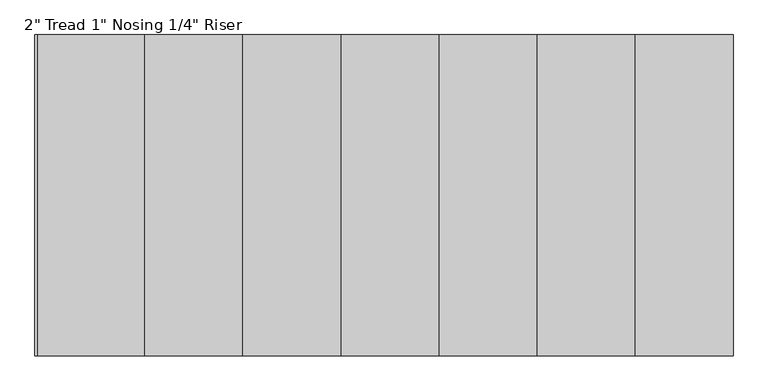
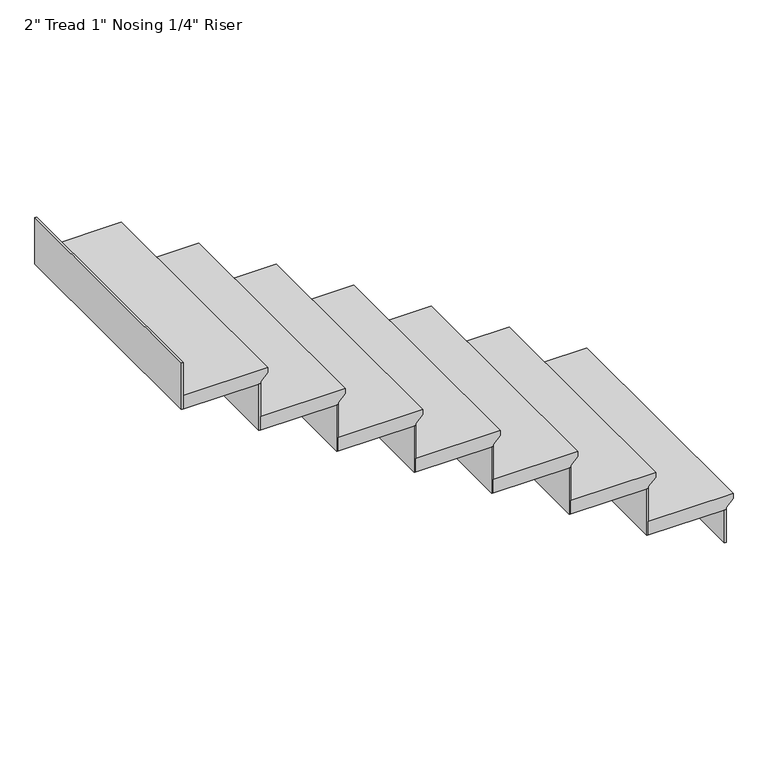
"""IFC4 building model written with IfcOpenShell, lengths in millimetres: stair flight geometry."""

from ifc_helpers import new_model, si_unit, origin, place, context, project, spatial, faceted_brep, source, transform, mapped, element, save


def stair_flight_80511569(model_context):
    return source(origin(), model_context, "Body", "Brep", [
        faceted_brep([(31519.2316163, 9282.3980552, 3968.75), (31519.2316163, 9282.3980552, 3987.8), (31519.2316163, 8367.9980552, 3987.8), (31519.2316163, 8367.9980552, 3968.75), (31493.8316163, 9282.3980552, 3943.35), (31493.8316163, 8367.9980552, 3943.35), (31214.4316163, 9282.3980552, 3987.8), (31214.4316163, 8367.9980552, 3987.8), (31493.8316163, 8367.9980552, 3937.0), (31214.4316163, 8367.9980552, 3937.0), (31214.4316163, 9282.3980552, 3937.0), (31493.8316163, 9282.3980552, 3937.0)], [[[0, 1, 2, 3]], [[4, 0, 3, 5]], [[2, 1, 6, 7]], [[8, 9, 10, 11]], [[2, 7, 9, 8, 5, 3]], [[8, 11, 4, 5]], [[6, 1, 0, 4, 11, 10]], [[7, 6, 10, 9]]]),
        faceted_brep([(31493.8316163, 9282.3980552, 3937.0), (31493.8316163, 9282.3980552, 3810.0), (31487.4816163, 9282.3980552, 3810.0), (31487.4816163, 9282.3980552, 3937.0), (31493.8316163, 8367.9980552, 3937.0), (31487.4816163, 8367.9980552, 3937.0), (31487.4816163, 8367.9980552, 3810.0), (31493.8316163, 8367.9980552, 3810.0)], [[[0, 1, 2, 3]], [[4, 5, 6, 7]], [[1, 0, 4, 7]], [[2, 1, 7, 6]], [[3, 2, 6, 5]], [[0, 3, 5, 4]]]),
        faceted_brep([(31214.4316163, 9282.3980552, 4114.8), (31214.4316163, 9282.3980552, 3937.0), (31208.0816163, 9282.3980552, 3937.0), (31208.0816163, 9282.3980552, 4114.8), (31214.4316163, 8367.9980552, 4114.8), (31208.0816163, 8367.9980552, 4114.8), (31208.0816163, 8367.9980552, 3937.0), (31214.4316163, 8367.9980552, 3937.0)], [[[0, 1, 2, 3]], [[4, 5, 6, 7]], [[1, 0, 4, 7]], [[2, 1, 7, 6]], [[3, 2, 6, 5]], [[0, 3, 5, 4]]]),
        faceted_brep([(31239.8316163, 8367.9980552, 4165.6), (31239.8316163, 9282.3980552, 4165.6), (30935.0316163, 9282.3980552, 4165.6), (30935.0316163, 8367.9980552, 4165.6), (31214.4316163, 8367.9980552, 4114.8), (30935.0316163, 8367.9980552, 4114.8), (30935.0316163, 9282.3980552, 4114.8), (31214.4316163, 9282.3980552, 4114.8), (31214.4316163, 8367.9980552, 4121.15), (31239.8316163, 8367.9980552, 4146.55), (31214.4316163, 9282.3980552, 4121.15), (31239.8316163, 9282.3980552, 4146.55)], [[[0, 1, 2, 3]], [[4, 5, 6, 7]], [[0, 3, 5, 4, 8, 9]], [[4, 7, 10, 8]], [[2, 1, 11, 10, 7, 6]], [[3, 2, 6, 5]], [[11, 1, 0, 9]], [[10, 11, 9, 8]]]),
        faceted_brep([(30935.0316163, 9282.3980552, 4292.6), (30935.0316163, 9282.3980552, 4114.8), (30928.6816163, 9282.3980552, 4114.8), (30928.6816163, 9282.3980552, 4292.6), (30935.0316163, 8367.9980552, 4292.6), (30928.6816163, 8367.9980552, 4292.6), (30928.6816163, 8367.9980552, 4114.8), (30935.0316163, 8367.9980552, 4114.8)], [[[0, 1, 2, 3]], [[4, 5, 6, 7]], [[1, 0, 4, 7]], [[2, 1, 7, 6]], [[3, 2, 6, 5]], [[0, 3, 5, 4]]]),
        faceted_brep([(30960.4316163, 8367.9980552, 4343.4), (30960.4316163, 9282.3980552, 4343.4), (30655.6316163, 9282.3980552, 4343.4), (30655.6316163, 8367.9980552, 4343.4), (30935.0316163, 8367.9980552, 4292.6), (30655.6316163, 8367.9980552, 4292.6), (30655.6316163, 9282.3980552, 4292.6), (30935.0316163, 9282.3980552, 4292.6), (30935.0316163, 8367.9980552, 4298.95), (30960.4316163, 8367.9980552, 4324.35), (30935.0316163, 9282.3980552, 4298.95), (30960.4316163, 9282.3980552, 4324.35)], [[[0, 1, 2, 3]], [[4, 5, 6, 7]], [[0, 3, 5, 4, 8, 9]], [[4, 7, 10, 8]], [[2, 1, 11, 10, 7, 6]], [[3, 2, 6, 5]], [[11, 1, 0, 9]], [[10, 11, 9, 8]]]),
        faceted_brep([(30655.6316163, 9282.3980552, 4470.4), (30655.6316163, 9282.3980552, 4292.6), (30649.2816163, 9282.3980552, 4292.6), (30649.2816163, 9282.3980552, 4470.4), (30655.6316163, 8367.9980552, 4470.4), (30649.2816163, 8367.9980552, 4470.4), (30649.2816163, 8367.9980552, 4292.6), (30655.6316163, 8367.9980552, 4292.6)], [[[0, 1, 2, 3]], [[4, 5, 6, 7]], [[1, 0, 4, 7]], [[2, 1, 7, 6]], [[3, 2, 6, 5]], [[0, 3, 5, 4]]]),
        faceted_brep([(30681.0316163, 8367.9980552, 4521.2), (30681.0316163, 9282.3980552, 4521.2), (30376.2316163, 9282.3980552, 4521.2), (30376.2316163, 8367.9980552, 4521.2), (30655.6316163, 8367.9980552, 4470.4), (30376.2316163, 8367.9980552, 4470.4), (30376.2316163, 9282.3980552, 4470.4), (30655.6316163, 9282.3980552, 4470.4), (30655.6316163, 8367.9980552, 4476.75), (30681.0316163, 8367.9980552, 4502.15), (30655.6316163, 9282.3980552, 4476.75), (30681.0316163, 9282.3980552, 4502.15)], [[[0, 1, 2, 3]], [[4, 5, 6, 7]], [[0, 3, 5, 4, 8, 9]], [[4, 7, 10, 8]], [[2, 1, 11, 10, 7, 6]], [[3, 2, 6, 5]], [[11, 1, 0, 9]], [[10, 11, 9, 8]]]),
        faceted_brep([(30376.2316163, 9282.3980552, 4648.2), (30376.2316163, 9282.3980552, 4470.4), (30369.8816163, 9282.3980552, 4470.4), (30369.8816163, 9282.3980552, 4648.2), (30376.2316163, 8367.9980552, 4648.2), (30369.8816163, 8367.9980552, 4648.2), (30369.8816163, 8367.9980552, 4470.4), (30376.2316163, 8367.9980552, 4470.4)], [[[0, 1, 2, 3]], [[4, 5, 6, 7]], [[1, 0, 4, 7]], [[2, 1, 7, 6]], [[3, 2, 6, 5]], [[0, 3, 5, 4]]]),
        faceted_brep([(30401.6316163, 8367.9980552, 4699.0), (30401.6316163, 9282.3980552, 4699.0), (30096.8316163, 9282.3980552, 4699.0), (30096.8316163, 8367.9980552, 4699.0), (30376.2316163, 8367.9980552, 4648.2), (30096.8316163, 8367.9980552, 4648.2), (30096.8316163, 9282.3980552, 4648.2), (30376.2316163, 9282.3980552, 4648.2), (30376.2316163, 8367.9980552, 4654.55), (30401.6316163, 8367.9980552, 4679.95), (30376.2316163, 9282.3980552, 4654.55), (30401.6316163, 9282.3980552, 4679.95)], [[[0, 1, 2, 3]], [[4, 5, 6, 7]], [[0, 3, 5, 4, 8, 9]], [[4, 7, 10, 8]], [[2, 1, 11, 10, 7, 6]], [[3, 2, 6, 5]], [[11, 1, 0, 9]], [[10, 11, 9, 8]]]),
        faceted_brep([(30096.8316163, 9282.3980552, 4826.0), (30096.8316163, 9282.3980552, 4648.2), (30090.4816163, 9282.3980552, 4648.2), (30090.4816163, 9282.3980552, 4826.0), (30096.8316163, 8367.9980552, 4826.0), (30090.4816163, 8367.9980552, 4826.0), (30090.4816163, 8367.9980552, 4648.2), (30096.8316163, 8367.9980552, 4648.2)], [[[0, 1, 2, 3]], [[4, 5, 6, 7]], [[1, 0, 4, 7]], [[2, 1, 7, 6]], [[3, 2, 6, 5]], [[0, 3, 5, 4]]]),
        faceted_brep([(30122.2316163, 8367.9980552, 4876.8), (30122.2316163, 9282.3980552, 4876.8), (29817.4316163, 9282.3980552, 4876.8), (29817.4316163, 8367.9980552, 4876.8), (30096.8316163, 8367.9980552, 4826.0), (29817.4316163, 8367.9980552, 4826.0), (29817.4316163, 9282.3980552, 4826.0), (30096.8316163, 9282.3980552, 4826.0), (30096.8316163, 8367.9980552, 4832.35), (30122.2316163, 8367.9980552, 4857.75), (30096.8316163, 9282.3980552, 4832.35), (30122.2316163, 9282.3980552, 4857.75)], [[[0, 1, 2, 3]], [[4, 5, 6, 7]], [[0, 3, 5, 4, 8, 9]], [[4, 7, 10, 8]], [[2, 1, 11, 10, 7, 6]], [[3, 2, 6, 5]], [[11, 1, 0, 9]], [[10, 11, 9, 8]]]),
        faceted_brep([(29538.0316163, 9282.3980552, 5181.6), (29538.0316163, 9282.3980552, 5003.8), (29531.6816163, 9282.3980552, 5003.8), (29531.6816163, 9282.3980552, 5181.6), (29538.0316163, 8367.9980552, 5181.6), (29531.6816163, 8367.9980552, 5181.6), (29531.6816163, 8367.9980552, 5003.8), (29538.0316163, 8367.9980552, 5003.8)], [[[0, 1, 2, 3]], [[4, 5, 6, 7]], [[1, 0, 4, 7]], [[2, 1, 7, 6]], [[3, 2, 6, 5]], [[0, 3, 5, 4]]]),
        faceted_brep([(29817.4316163, 9282.3980552, 5003.8), (29817.4316163, 9282.3980552, 4826.0), (29811.0816163, 9282.3980552, 4826.0), (29811.0816163, 9282.3980552, 5003.8), (29817.4316163, 8367.9980552, 5003.8), (29811.0816163, 8367.9980552, 5003.8), (29811.0816163, 8367.9980552, 4826.0), (29817.4316163, 8367.9980552, 4826.0)], [[[0, 1, 2, 3]], [[4, 5, 6, 7]], [[1, 0, 4, 7]], [[2, 1, 7, 6]], [[3, 2, 6, 5]], [[0, 3, 5, 4]]]),
        faceted_brep([(29842.8316163, 8367.9980552, 5054.6), (29842.8316163, 9282.3980552, 5054.6), (29563.4316163, 9282.3980552, 5054.6), (29538.0316163, 9282.3980552, 5054.6), (29538.0316163, 8367.9980552, 5054.6), (29817.4316163, 8367.9980552, 5003.8), (29538.0316163, 8367.9980552, 5003.8), (29538.0316163, 9282.3980552, 5003.8), (29563.4316163, 9282.3980552, 5003.8), (29817.4316163, 9282.3980552, 5003.8), (29817.4316163, 8367.9980552, 5010.15), (29842.8316163, 8367.9980552, 5035.55), (29817.4316163, 9282.3980552, 5010.15), (29842.8316163, 9282.3980552, 5035.55)], [[[0, 1, 2, 3, 4]], [[5, 6, 7, 8, 9]], [[0, 4, 6, 5, 10, 11]], [[5, 9, 12, 10]], [[2, 1, 13, 12, 9, 8]], [[3, 2, 8, 7]], [[4, 3, 7, 6]], [[13, 1, 0, 11]], [[12, 13, 11, 10]]]),
    ])


if __name__ == "__main__":
    model = new_model("IFC4")
    model_context = context("Model", 3, world=origin())
    ifc_project = project(units=[si_unit("LENGTHUNIT", "METRE", prefix="MILLI")], contexts=[model_context])
    site = spatial("IfcSite", under=ifc_project)
    building = spatial("IfcBuilding", under=site)
    placement = place(None, origin())
    stair_flight_shape = stair_flight_80511569(model_context)
    element("IfcStairFlight", 1, ObjectType="2\" Tread 1\" Nosing 1/4\" Riser", at=placement, inside=building, context=model_context, shape_type="MappedRepresentation", body=[
        mapped(stair_flight_shape, transform((0.0, 0.0, 0.0), x_axis=(1.0, 0.0, 0.0), y_axis=(0.0, 1.0, 0.0), z_axis=(0.0, 0.0, 1.0))),
    ])
    save(model, "model.ifc")
